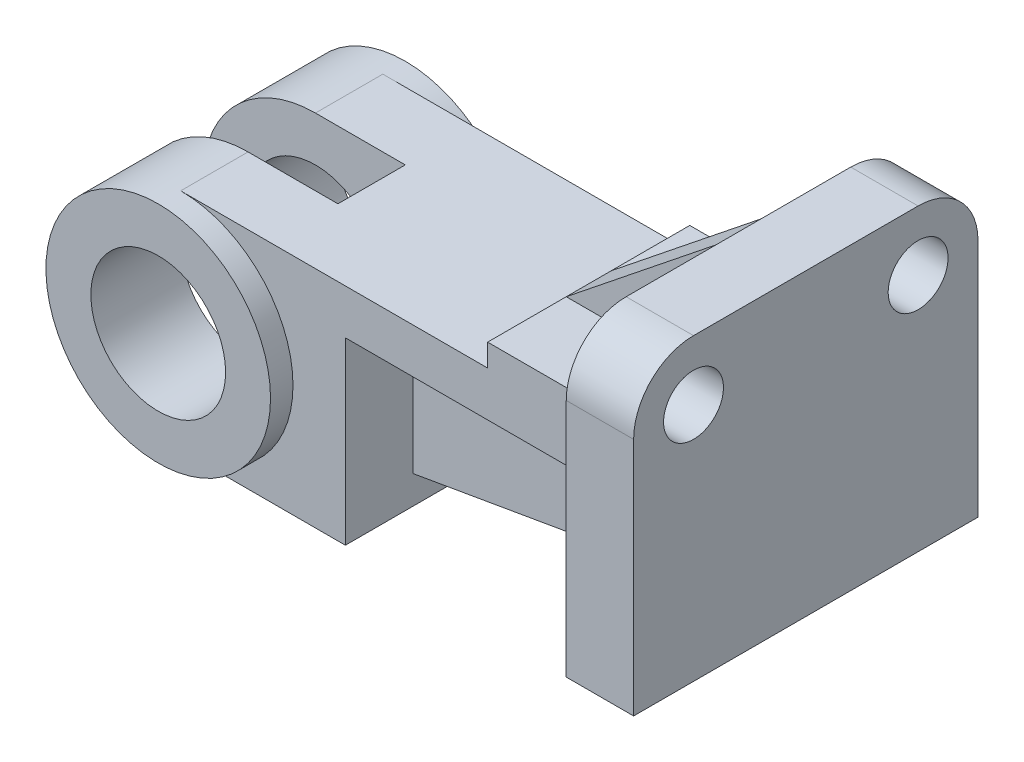
ISO-10303-21;
HEADER;
FILE_DESCRIPTION(('STEP AP214'),'2;1');
FILE_NAME('part.step','',(''),(''),'','','');
FILE_SCHEMA(('AUTOMOTIVE_DESIGN { 1 0 10303 214 1 1 1 1 }'));
ENDSEC;
DATA;
#1=APPLICATION_CONTEXT('core data for automotive mechanical design processes');
#2=APPLICATION_PROTOCOL_DEFINITION('international standard','automotive_design',2000,#1);
#3=PRODUCT_CONTEXT('',#1,'mechanical');
#4=PRODUCT('Part','Part','',(#3));
#5=PRODUCT_RELATED_PRODUCT_CATEGORY('part','',(#4));
#6=PRODUCT_DEFINITION_FORMATION('','',#4);
#7=PRODUCT_DEFINITION_CONTEXT('part definition',#1,'design');
#8=PRODUCT_DEFINITION('design','',#6,#7);
#9=PRODUCT_DEFINITION_SHAPE('','',#8);
#10=(LENGTH_UNIT() NAMED_UNIT(*) SI_UNIT(.MILLI.,.METRE.));
#11=(NAMED_UNIT(*) PLANE_ANGLE_UNIT() SI_UNIT($,.RADIAN.));
#12=(NAMED_UNIT(*) SI_UNIT($,.STERADIAN.) SOLID_ANGLE_UNIT());
#13=UNCERTAINTY_MEASURE_WITH_UNIT(LENGTH_MEASURE(1.E-05),#10,'distance_accuracy_value','');
#14=(GEOMETRIC_REPRESENTATION_CONTEXT(3) GLOBAL_UNCERTAINTY_ASSIGNED_CONTEXT((#13)) GLOBAL_UNIT_ASSIGNED_CONTEXT((#10,
#11,#12)) REPRESENTATION_CONTEXT('',''));
#15=CARTESIAN_POINT('',(0.,0.,0.));
#16=DIRECTION('',(0.,0.,1.));
#17=DIRECTION('',(1.,0.,0.));
#18=AXIS2_PLACEMENT_3D('',#15,#16,#17);
#19=CARTESIAN_POINT('',(104.,0.,-74.));
#20=DIRECTION('',(-1.,0.,0.));
#21=DIRECTION('',(0.,0.,1.));
#22=AXIS2_PLACEMENT_3D('',#19,#20,#21);
#23=PLANE('',#22);
#24=DIRECTION('',(0.,0.,1.));
#25=VECTOR('',#24,1.);
#26=CARTESIAN_POINT('',(104.,18.,-74.));
#27=LINE('',#26,#25);
#28=CARTESIAN_POINT('',(104.,18.,0.));
#29=VERTEX_POINT('',#28);
#30=CARTESIAN_POINT('',(104.,18.,18.));
#31=VERTEX_POINT('',#30);
#32=EDGE_CURVE('E277',#29,#31,#27,.T.);
#33=ORIENTED_EDGE('',*,*,#32,.F.);
#34=DIRECTION('',(0.,-1.,0.));
#35=VECTOR('',#34,1.);
#36=CARTESIAN_POINT('',(104.,0.,0.));
#37=LINE('',#36,#35);
#38=CARTESIAN_POINT('',(104.,-12.,0.));
#39=VERTEX_POINT('',#38);
#40=EDGE_CURVE('E57',#29,#39,#37,.T.);
#41=ORIENTED_EDGE('',*,*,#40,.T.);
#42=DIRECTION('',(0.,0.,1.));
#43=VECTOR('',#42,1.);
#44=CARTESIAN_POINT('',(104.,-12.,-74.));
#45=LINE('',#44,#43);
#46=CARTESIAN_POINT('',(104.,-12.,18.));
#47=VERTEX_POINT('',#46);
#48=EDGE_CURVE('E284',#39,#47,#45,.T.);
#49=ORIENTED_EDGE('',*,*,#48,.T.);
#50=DIRECTION('',(0.,-1.,0.));
#51=VECTOR('',#50,1.);
#52=CARTESIAN_POINT('',(104.,0.,18.));
#53=LINE('',#52,#51);
#54=EDGE_CURVE('E263',#31,#47,#53,.T.);
#55=ORIENTED_EDGE('',*,*,#54,.F.);
#56=EDGE_LOOP('',(#33,#41,#49,#55));
#57=FACE_BOUND('',#56,.T.);
#58=ADVANCED_FACE('F37',(#57),#23,.T.);
#59=CARTESIAN_POINT('',(0.,18.,-74.));
#60=DIRECTION('',(0.,-1.,0.));
#61=DIRECTION('',(0.,0.,-1.));
#62=AXIS2_PLACEMENT_3D('',#59,#60,#61);
#63=PLANE('',#62);
#64=DIRECTION('',(0.,0.,1.));
#65=VECTOR('',#64,1.);
#66=CARTESIAN_POINT('',(44.,18.,-74.));
#67=LINE('',#66,#65);
#68=CARTESIAN_POINT('',(44.,18.,0.));
#69=VERTEX_POINT('',#68);
#70=CARTESIAN_POINT('',(44.,18.,18.));
#71=VERTEX_POINT('',#70);
#72=EDGE_CURVE('E286',#69,#71,#67,.T.);
#73=ORIENTED_EDGE('',*,*,#72,.F.);
#74=DIRECTION('',(1.,0.,0.));
#75=VECTOR('',#74,1.);
#76=CARTESIAN_POINT('',(0.,18.,0.));
#77=LINE('',#76,#75);
#78=EDGE_CURVE('E232',#69,#29,#77,.T.);
#79=ORIENTED_EDGE('',*,*,#78,.T.);
#80=ORIENTED_EDGE('',*,*,#32,.T.);
#81=DIRECTION('',(1.,0.,0.));
#82=VECTOR('',#81,1.);
#83=CARTESIAN_POINT('',(0.,18.,18.));
#84=LINE('',#83,#82);
#85=EDGE_CURVE('E267',#71,#31,#84,.T.);
#86=ORIENTED_EDGE('',*,*,#85,.F.);
#87=EDGE_LOOP('',(#73,#79,#80,#86));
#88=FACE_BOUND('',#87,.T.);
#89=ADVANCED_FACE('F496',(#88),#63,.T.);
#90=CARTESIAN_POINT('',(122.,-30.,-36.));
#91=DIRECTION('',(0.,-1.,0.));
#92=DIRECTION('',(0.,0.,-1.));
#93=AXIS2_PLACEMENT_3D('',#90,#91,#92);
#94=PLANE('',#93);
#95=DIRECTION('',(1.,0.,0.));
#96=VECTOR('',#95,1.);
#97=CARTESIAN_POINT('',(122.,-30.,-36.));
#98=LINE('',#97,#96);
#99=CARTESIAN_POINT('',(0.,-30.,-36.));
#100=VERTEX_POINT('',#99);
#101=CARTESIAN_POINT('',(44.,-30.,-36.));
#102=VERTEX_POINT('',#101);
#103=EDGE_CURVE('E416',#100,#102,#98,.T.);
#104=ORIENTED_EDGE('',*,*,#103,.T.);
#105=DIRECTION('',(0.,0.,1.));
#106=VECTOR('',#105,1.);
#107=CARTESIAN_POINT('',(44.,-30.,-74.));
#108=LINE('',#107,#106);
#109=CARTESIAN_POINT('',(44.,-30.,18.));
#110=VERTEX_POINT('',#109);
#111=EDGE_CURVE('E281',#102,#110,#108,.T.);
#112=ORIENTED_EDGE('',*,*,#111,.T.);
#113=DIRECTION('',(1.,0.,0.));
#114=VECTOR('',#113,1.);
#115=CARTESIAN_POINT('',(122.,-30.,18.));
#116=LINE('',#115,#114);
#117=CARTESIAN_POINT('',(0.,-30.,18.));
#118=VERTEX_POINT('',#117);
#119=EDGE_CURVE('E426',#118,#110,#116,.T.);
#120=ORIENTED_EDGE('',*,*,#119,.F.);
#121=DIRECTION('',(0.,0.,1.));
#122=VECTOR('',#121,1.);
#123=CARTESIAN_POINT('',(0.,-30.,-36.));
#124=LINE('',#123,#122);
#125=CARTESIAN_POINT('',(0.,-30.,0.));
#126=VERTEX_POINT('',#125);
#127=EDGE_CURVE('E424',#126,#118,#124,.T.);
#128=ORIENTED_EDGE('',*,*,#127,.F.);
#129=DIRECTION('',(-1.,0.,0.));
#130=VECTOR('',#129,1.);
#131=CARTESIAN_POINT('',(122.,-30.,0.));
#132=LINE('',#131,#130);
#133=CARTESIAN_POINT('',(24.,-30.,0.));
#134=VERTEX_POINT('',#133);
#135=EDGE_CURVE('E446',#134,#126,#132,.T.);
#136=ORIENTED_EDGE('',*,*,#135,.F.);
#137=DIRECTION('',(0.,0.,1.));
#138=VECTOR('',#137,1.);
#139=CARTESIAN_POINT('',(24.,-30.,-36.));
#140=LINE('',#139,#138);
#141=CARTESIAN_POINT('',(24.,-30.,-18.));
#142=VERTEX_POINT('',#141);
#143=EDGE_CURVE('E397',#142,#134,#140,.T.);
#144=ORIENTED_EDGE('',*,*,#143,.F.);
#145=DIRECTION('',(1.,0.,0.));
#146=VECTOR('',#145,1.);
#147=CARTESIAN_POINT('',(122.,-30.,-18.));
#148=LINE('',#147,#146);
#149=CARTESIAN_POINT('',(0.,-30.,-18.));
#150=VERTEX_POINT('',#149);
#151=EDGE_CURVE('E395',#150,#142,#148,.T.);
#152=ORIENTED_EDGE('',*,*,#151,.F.);
#153=EDGE_CURVE('E439',#100,#150,#124,.T.);
#154=ORIENTED_EDGE('',*,*,#153,.F.);
#155=EDGE_LOOP('',(#104,#112,#120,#128,#136,#144,#152,#154));
#156=FACE_BOUND('',#155,.T.);
#157=ADVANCED_FACE('F502',(#156),#94,.T.);
#158=CARTESIAN_POINT('',(0.,36.,0.));
#159=DIRECTION('',(0.,-1.,0.));
#160=DIRECTION('',(0.,0.,-1.));
#161=AXIS2_PLACEMENT_3D('',#158,#159,#160);
#162=PLANE('',#161);
#163=DIRECTION('',(0.,0.,1.));
#164=VECTOR('',#163,1.);
#165=CARTESIAN_POINT('',(82.,36.,18.));
#166=LINE('',#165,#164);
#167=CARTESIAN_POINT('',(82.,36.,-3.));
#168=VERTEX_POINT('',#167);
#169=CARTESIAN_POINT('',(82.,36.,18.));
#170=VERTEX_POINT('',#169);
#171=EDGE_CURVE('E359',#168,#170,#166,.T.);
#172=ORIENTED_EDGE('',*,*,#171,.T.);
#173=DIRECTION('',(1.,0.,0.));
#174=VECTOR('',#173,1.);
#175=CARTESIAN_POINT('',(122.,36.,18.));
#176=LINE('',#175,#174);
#177=CARTESIAN_POINT('',(122.,36.,18.));
#178=VERTEX_POINT('',#177);
#179=EDGE_CURVE('E361',#170,#178,#176,.T.);
#180=ORIENTED_EDGE('',*,*,#179,.T.);
#181=DIRECTION('',(0.,0.,-1.));
#182=VECTOR('',#181,1.);
#183=CARTESIAN_POINT('',(122.,36.,-36.));
#184=LINE('',#183,#182);
#185=CARTESIAN_POINT('',(122.,36.,-3.));
#186=VERTEX_POINT('',#185);
#187=EDGE_CURVE('E355',#178,#186,#184,.T.);
#188=ORIENTED_EDGE('',*,*,#187,.T.);
#189=DIRECTION('',(1.,0.,0.));
#190=VECTOR('',#189,1.);
#191=CARTESIAN_POINT('',(0.,36.,-3.));
#192=LINE('',#191,#190);
#193=EDGE_CURVE('E302',#168,#186,#192,.T.);
#194=ORIENTED_EDGE('',*,*,#193,.F.);
#195=EDGE_LOOP('',(#172,#180,#188,#194));
#196=FACE_BOUND('',#195,.T.);
#197=ADVANCED_FACE('F611',(#196),#162,.F.);
#198=CARTESIAN_POINT('',(122.,-12.,-55.));
#199=DIRECTION('',(1.,0.,0.));
#200=DIRECTION('',(0.,0.,-1.));
#201=AXIS2_PLACEMENT_3D('',#198,#199,#200);
#202=PLANE('',#201);
#203=DIRECTION('',(0.,1.,0.));
#204=VECTOR('',#203,1.);
#205=CARTESIAN_POINT('',(122.,-12.,-3.));
#206=LINE('',#205,#204);
#207=CARTESIAN_POINT('',(122.,68.,-3.));
#208=VERTEX_POINT('',#207);
#209=EDGE_CURVE('E301',#186,#208,#206,.T.);
#210=ORIENTED_EDGE('',*,*,#209,.F.);
#211=ORIENTED_EDGE('',*,*,#187,.F.);
#212=DIRECTION('',(0.,1.,0.));
#213=VECTOR('',#212,1.);
#214=CARTESIAN_POINT('',(122.,30.,18.));
#215=LINE('',#214,#213);
#216=CARTESIAN_POINT('',(122.,-12.,18.));
#217=VERTEX_POINT('',#216);
#218=EDGE_CURVE('E431',#217,#178,#215,.T.);
#219=ORIENTED_EDGE('',*,*,#218,.F.);
#220=DIRECTION('',(0.,0.,1.));
#221=VECTOR('',#220,1.);
#222=CARTESIAN_POINT('',(122.,-12.,-55.));
#223=LINE('',#222,#221);
#224=CARTESIAN_POINT('',(122.,-12.,37.));
#225=VERTEX_POINT('',#224);
#226=EDGE_CURVE('E347',#217,#225,#223,.T.);
#227=ORIENTED_EDGE('',*,*,#226,.T.);
#228=DIRECTION('',(0.,1.,0.));
#229=VECTOR('',#228,1.);
#230=CARTESIAN_POINT('',(122.,-12.,37.));
#231=LINE('',#230,#229);
#232=CARTESIAN_POINT('',(122.,52.,37.));
#233=VERTEX_POINT('',#232);
#234=EDGE_CURVE('E336',#225,#233,#231,.T.);
#235=ORIENTED_EDGE('',*,*,#234,.T.);
#236=CARTESIAN_POINT('',(122.,52.,21.));
#237=DIRECTION('',(1.,0.,0.));
#238=DIRECTION('',(0.,0.,-1.));
#239=AXIS2_PLACEMENT_3D('',#236,#237,#238);
#240=CIRCLE('',#239,16.);
#241=CARTESIAN_POINT('',(122.,68.,21.));
#242=VERTEX_POINT('',#241);
#243=EDGE_CURVE('E463',#233,#242,#240,.F.);
#244=ORIENTED_EDGE('',*,*,#243,.T.);
#245=DIRECTION('',(0.,0.,1.));
#246=VECTOR('',#245,1.);
#247=CARTESIAN_POINT('',(122.,68.,-55.));
#248=LINE('',#247,#246);
#249=EDGE_CURVE('E346',#208,#242,#248,.T.);
#250=ORIENTED_EDGE('',*,*,#249,.F.);
#251=EDGE_LOOP('',(#210,#211,#219,#227,#235,#244,#250));
#252=FACE_BOUND('',#251,.T.);
#253=CARTESIAN_POINT('',(122.,52.,21.));
#254=DIRECTION('',(-1.,0.,0.));
#255=DIRECTION('',(0.,0.,1.));
#256=AXIS2_PLACEMENT_3D('',#253,#254,#255);
#257=CIRCLE('',#256,8.);
#258=CARTESIAN_POINT('',(122.,52.,29.));
#259=VERTEX_POINT('',#258);
#260=EDGE_CURVE('E316',#259,#259,#257,.T.);
#261=ORIENTED_EDGE('',*,*,#260,.F.);
#262=EDGE_LOOP('',(#261));
#263=FACE_BOUND('',#262,.T.);
#264=ADVANCED_FACE('F642',(#252,#263),#202,.F.);
#265=CARTESIAN_POINT('',(0.,30.,-36.));
#266=DIRECTION('',(0.,1.,0.));
#267=DIRECTION('',(0.,0.,1.));
#268=AXIS2_PLACEMENT_3D('',#265,#266,#267);
#269=PLANE('',#268);
#270=DIRECTION('',(-1.,0.,0.));
#271=VECTOR('',#270,1.);
#272=CARTESIAN_POINT('',(24.,30.,-18.));
#273=LINE('',#272,#271);
#274=CARTESIAN_POINT('',(24.,30.,-18.));
#275=VERTEX_POINT('',#274);
#276=CARTESIAN_POINT('',(0.,30.,-18.));
#277=VERTEX_POINT('',#276);
#278=EDGE_CURVE('E389',#275,#277,#273,.T.);
#279=ORIENTED_EDGE('',*,*,#278,.F.);
#280=DIRECTION('',(0.,0.,-1.));
#281=VECTOR('',#280,1.);
#282=CARTESIAN_POINT('',(24.,30.,0.));
#283=LINE('',#282,#281);
#284=CARTESIAN_POINT('',(24.,30.,0.));
#285=VERTEX_POINT('',#284);
#286=EDGE_CURVE('E383',#285,#275,#283,.T.);
#287=ORIENTED_EDGE('',*,*,#286,.F.);
#288=DIRECTION('',(1.,0.,0.));
#289=VECTOR('',#288,1.);
#290=CARTESIAN_POINT('',(0.,30.,0.));
#291=LINE('',#290,#289);
#292=CARTESIAN_POINT('',(0.,30.,0.));
#293=VERTEX_POINT('',#292);
#294=EDGE_CURVE('E385',#293,#285,#291,.T.);
#295=ORIENTED_EDGE('',*,*,#294,.F.);
#296=DIRECTION('',(0.,0.,1.));
#297=VECTOR('',#296,1.);
#298=CARTESIAN_POINT('',(0.,30.,-36.));
#299=LINE('',#298,#297);
#300=CARTESIAN_POINT('',(0.,30.,18.));
#301=VERTEX_POINT('',#300);
#302=EDGE_CURVE('E437',#293,#301,#299,.T.);
#303=ORIENTED_EDGE('',*,*,#302,.T.);
#304=DIRECTION('',(-1.,0.,0.));
#305=VECTOR('',#304,1.);
#306=CARTESIAN_POINT('',(0.,30.,18.));
#307=LINE('',#306,#305);
#308=CARTESIAN_POINT('',(82.,30.,18.));
#309=VERTEX_POINT('',#308);
#310=EDGE_CURVE('E417',#309,#301,#307,.T.);
#311=ORIENTED_EDGE('',*,*,#310,.F.);
#312=DIRECTION('',(0.,0.,1.));
#313=VECTOR('',#312,1.);
#314=CARTESIAN_POINT('',(82.,30.,18.));
#315=LINE('',#314,#313);
#316=CARTESIAN_POINT('',(82.,30.,-36.));
#317=VERTEX_POINT('',#316);
#318=EDGE_CURVE('E353',#317,#309,#315,.T.);
#319=ORIENTED_EDGE('',*,*,#318,.F.);
#320=DIRECTION('',(-1.,0.,0.));
#321=VECTOR('',#320,1.);
#322=CARTESIAN_POINT('',(0.,30.,-36.));
#323=LINE('',#322,#321);
#324=CARTESIAN_POINT('',(0.,30.,-36.));
#325=VERTEX_POINT('',#324);
#326=EDGE_CURVE('E421',#317,#325,#323,.T.);
#327=ORIENTED_EDGE('',*,*,#326,.T.);
#328=EDGE_CURVE('E434',#325,#277,#299,.T.);
#329=ORIENTED_EDGE('',*,*,#328,.T.);
#330=EDGE_LOOP('',(#279,#287,#295,#303,#311,#319,#327,#329));
#331=FACE_BOUND('',#330,.T.);
#332=ADVANCED_FACE('F646',(#331),#269,.T.);
#333=CARTESIAN_POINT('',(0.,0.,0.));
#334=DIRECTION('',(0.,0.,1.));
#335=DIRECTION('',(1.,0.,0.));
#336=AXIS2_PLACEMENT_3D('',#333,#334,#335);
#337=PLANE('',#336);
#338=ORIENTED_EDGE('',*,*,#135,.T.);
#339=CARTESIAN_POINT('',(0.,0.,0.));
#340=DIRECTION('',(0.,0.,1.));
#341=DIRECTION('',(1.,0.,0.));
#342=AXIS2_PLACEMENT_3D('',#339,#340,#341);
#343=CIRCLE('',#342,30.);
#344=EDGE_CURVE('E448',#293,#126,#343,.T.);
#345=ORIENTED_EDGE('',*,*,#344,.F.);
#346=ORIENTED_EDGE('',*,*,#294,.T.);
#347=DIRECTION('',(0.,1.,0.));
#348=VECTOR('',#347,1.);
#349=CARTESIAN_POINT('',(24.,-66.,0.));
#350=LINE('',#349,#348);
#351=EDGE_CURVE('E388',#134,#285,#350,.T.);
#352=ORIENTED_EDGE('',*,*,#351,.F.);
#353=EDGE_LOOP('',(#338,#345,#346,#352));
#354=FACE_BOUND('',#353,.T.);
#355=CARTESIAN_POINT('',(0.,0.,0.));
#356=DIRECTION('',(0.,0.,1.));
#357=DIRECTION('',(1.,0.,0.));
#358=AXIS2_PLACEMENT_3D('',#355,#356,#357);
#359=CIRCLE('',#358,18.);
#360=CARTESIAN_POINT('',(18.,0.,0.));
#361=VERTEX_POINT('',#360);
#362=EDGE_CURVE('E444',#361,#361,#359,.T.);
#363=ORIENTED_EDGE('',*,*,#362,.T.);
#364=EDGE_LOOP('',(#363));
#365=FACE_BOUND('',#364,.T.);
#366=ADVANCED_FACE('F747',(#354,#365),#337,.F.);
#367=CARTESIAN_POINT('',(0.,0.,-18.));
#368=DIRECTION('',(0.,0.,-1.));
#369=DIRECTION('',(-1.,0.,0.));
#370=AXIS2_PLACEMENT_3D('',#367,#368,#369);
#371=PLANE('',#370);
#372=CARTESIAN_POINT('',(0.,0.,-18.));
#373=DIRECTION('',(0.,0.,-1.));
#374=DIRECTION('',(-1.,0.,0.));
#375=AXIS2_PLACEMENT_3D('',#372,#373,#374);
#376=CIRCLE('',#375,18.);
#377=CARTESIAN_POINT('',(-18.,0.,-18.));
#378=VERTEX_POINT('',#377);
#379=EDGE_CURVE('E398',#378,#378,#376,.T.);
#380=ORIENTED_EDGE('',*,*,#379,.T.);
#381=EDGE_LOOP('',(#380));
#382=FACE_BOUND('',#381,.T.);
#383=CARTESIAN_POINT('',(0.,0.,-18.));
#384=DIRECTION('',(0.,0.,-1.));
#385=DIRECTION('',(-1.,0.,0.));
#386=AXIS2_PLACEMENT_3D('',#383,#384,#385);
#387=CIRCLE('',#386,30.);
#388=EDGE_CURVE('E401',#150,#277,#387,.T.);
#389=ORIENTED_EDGE('',*,*,#388,.F.);
#390=ORIENTED_EDGE('',*,*,#151,.T.);
#391=DIRECTION('',(0.,1.,0.));
#392=VECTOR('',#391,1.);
#393=CARTESIAN_POINT('',(24.,-66.,-18.));
#394=LINE('',#393,#392);
#395=EDGE_CURVE('E394',#142,#275,#394,.T.);
#396=ORIENTED_EDGE('',*,*,#395,.T.);
#397=ORIENTED_EDGE('',*,*,#278,.T.);
#398=EDGE_LOOP('',(#389,#390,#396,#397));
#399=FACE_BOUND('',#398,.T.);
#400=ADVANCED_FACE('F769',(#382,#399),#371,.F.);
#401=CARTESIAN_POINT('',(0.,0.,24.));
#402=DIRECTION('',(0.,0.,-1.));
#403=DIRECTION('',(-1.,0.,0.));
#404=AXIS2_PLACEMENT_3D('',#401,#402,#403);
#405=CYLINDRICAL_SURFACE('',#404,30.);
#406=CARTESIAN_POINT('',(0.,0.,18.));
#407=DIRECTION('',(0.,0.,-1.));
#408=DIRECTION('',(1.,0.,0.));
#409=AXIS2_PLACEMENT_3D('',#406,#407,#408);
#410=CIRCLE('',#409,30.);
#411=EDGE_CURVE('E410',#301,#118,#410,.T.);
#412=ORIENTED_EDGE('',*,*,#411,.F.);
#413=ORIENTED_EDGE('',*,*,#302,.F.);
#414=ORIENTED_EDGE('',*,*,#344,.T.);
#415=ORIENTED_EDGE('',*,*,#127,.T.);
#416=EDGE_LOOP('',(#412,#413,#414,#415));
#417=FACE_BOUND('',#416,.T.);
#418=CARTESIAN_POINT('',(0.,0.,24.));
#419=DIRECTION('',(0.,0.,1.));
#420=DIRECTION('',(1.,0.,0.));
#421=AXIS2_PLACEMENT_3D('',#418,#419,#420);
#422=CIRCLE('',#421,30.);
#423=CARTESIAN_POINT('',(30.,0.,24.));
#424=VERTEX_POINT('',#423);
#425=EDGE_CURVE('E447',#424,#424,#422,.T.);
#426=ORIENTED_EDGE('',*,*,#425,.F.);
#427=EDGE_LOOP('',(#426));
#428=FACE_BOUND('',#427,.T.);
#429=ADVANCED_FACE('F785',(#417,#428),#405,.T.);
#430=CARTESIAN_POINT('',(0.,0.,24.));
#431=DIRECTION('',(0.,0.,1.));
#432=DIRECTION('',(1.,0.,0.));
#433=AXIS2_PLACEMENT_3D('',#430,#431,#432);
#434=PLANE('',#433);
#435=CARTESIAN_POINT('',(0.,0.,24.));
#436=DIRECTION('',(0.,0.,1.));
#437=DIRECTION('',(1.,0.,0.));
#438=AXIS2_PLACEMENT_3D('',#435,#436,#437);
#439=CIRCLE('',#438,18.);
#440=CARTESIAN_POINT('',(18.,0.,24.));
#441=VERTEX_POINT('',#440);
#442=EDGE_CURVE('E438',#441,#441,#439,.T.);
#443=ORIENTED_EDGE('',*,*,#442,.F.);
#444=EDGE_LOOP('',(#443));
#445=FACE_BOUND('',#444,.T.);
#446=ORIENTED_EDGE('',*,*,#425,.T.);
#447=EDGE_LOOP('',(#446));
#448=FACE_BOUND('',#447,.T.);
#449=ADVANCED_FACE('F870',(#445,#448),#434,.T.);
#450=CARTESIAN_POINT('',(0.,0.,-74.));
#451=DIRECTION('',(0.,0.,1.));
#452=DIRECTION('',(1.,0.,0.));
#453=AXIS2_PLACEMENT_3D('',#450,#451,#452);
#454=CYLINDRICAL_SURFACE('',#453,18.);
#455=ORIENTED_EDGE('',*,*,#442,.T.);
#456=EDGE_LOOP('',(#455));
#457=FACE_BOUND('',#456,.T.);
#458=ORIENTED_EDGE('',*,*,#362,.F.);
#459=EDGE_LOOP('',(#458));
#460=FACE_BOUND('',#459,.T.);
#461=ADVANCED_FACE('F814',(#457,#460),#454,.F.);
#462=CARTESIAN_POINT('',(0.,0.,-36.));
#463=DIRECTION('',(0.,0.,1.));
#464=DIRECTION('',(1.,0.,0.));
#465=AXIS2_PLACEMENT_3D('',#462,#463,#464);
#466=PLANE('',#465);
#467=DIRECTION('',(0.,1.,0.));
#468=VECTOR('',#467,1.);
#469=CARTESIAN_POINT('',(122.,30.,-36.));
#470=LINE('',#469,#468);
#471=CARTESIAN_POINT('',(122.,-12.,-36.));
#472=VERTEX_POINT('',#471);
#473=CARTESIAN_POINT('',(122.,36.,-36.));
#474=VERTEX_POINT('',#473);
#475=EDGE_CURVE('E420',#472,#474,#470,.T.);
#476=ORIENTED_EDGE('',*,*,#475,.F.);
#477=DIRECTION('',(-1.,0.,0.));
#478=VECTOR('',#477,1.);
#479=CARTESIAN_POINT('',(0.,-12.,-36.));
#480=LINE('',#479,#478);
#481=CARTESIAN_POINT('',(104.,-12.,-36.));
#482=VERTEX_POINT('',#481);
#483=EDGE_CURVE('E278',#472,#482,#480,.T.);
#484=ORIENTED_EDGE('',*,*,#483,.T.);
#485=DIRECTION('',(0.,-1.,0.));
#486=VECTOR('',#485,1.);
#487=CARTESIAN_POINT('',(104.,0.,-36.));
#488=LINE('',#487,#486);
#489=CARTESIAN_POINT('',(104.,18.,-36.));
#490=VERTEX_POINT('',#489);
#491=EDGE_CURVE('E298',#490,#482,#488,.T.);
#492=ORIENTED_EDGE('',*,*,#491,.F.);
#493=DIRECTION('',(1.,0.,0.));
#494=VECTOR('',#493,1.);
#495=CARTESIAN_POINT('',(0.,18.,-36.));
#496=LINE('',#495,#494);
#497=CARTESIAN_POINT('',(44.,18.,-36.));
#498=VERTEX_POINT('',#497);
#499=EDGE_CURVE('E292',#498,#490,#496,.T.);
#500=ORIENTED_EDGE('',*,*,#499,.F.);
#501=DIRECTION('',(0.,1.,0.));
#502=VECTOR('',#501,1.);
#503=CARTESIAN_POINT('',(44.,0.,-36.));
#504=LINE('',#503,#502);
#505=EDGE_CURVE('E295',#102,#498,#504,.T.);
#506=ORIENTED_EDGE('',*,*,#505,.F.);
#507=ORIENTED_EDGE('',*,*,#103,.F.);
#508=CARTESIAN_POINT('',(0.,0.,-36.));
#509=DIRECTION('',(0.,0.,-1.));
#510=DIRECTION('',(1.,0.,0.));
#511=AXIS2_PLACEMENT_3D('',#508,#509,#510);
#512=CIRCLE('',#511,30.);
#513=EDGE_CURVE('E415',#325,#100,#512,.T.);
#514=ORIENTED_EDGE('',*,*,#513,.F.);
#515=ORIENTED_EDGE('',*,*,#326,.F.);
#516=DIRECTION('',(0.,-1.,0.));
#517=VECTOR('',#516,1.);
#518=CARTESIAN_POINT('',(82.,36.,-36.));
#519=LINE('',#518,#517);
#520=CARTESIAN_POINT('',(82.,36.,-36.));
#521=VERTEX_POINT('',#520);
#522=EDGE_CURVE('E369',#521,#317,#519,.T.);
#523=ORIENTED_EDGE('',*,*,#522,.F.);
#524=DIRECTION('',(-1.,0.,0.));
#525=VECTOR('',#524,1.);
#526=CARTESIAN_POINT('',(82.,36.,-36.));
#527=LINE('',#526,#525);
#528=EDGE_CURVE('E357',#474,#521,#527,.T.);
#529=ORIENTED_EDGE('',*,*,#528,.F.);
#530=EDGE_LOOP('',(#476,#484,#492,#500,#506,#507,#514,#515,#523,#529));
#531=FACE_BOUND('',#530,.T.);
#532=ADVANCED_FACE('F530',(#531),#466,.F.);
#533=CARTESIAN_POINT('',(0.,0.,18.));
#534=DIRECTION('',(0.,0.,1.));
#535=DIRECTION('',(1.,0.,0.));
#536=AXIS2_PLACEMENT_3D('',#533,#534,#535);
#537=PLANE('',#536);
#538=DIRECTION('',(-1.,0.,0.));
#539=VECTOR('',#538,1.);
#540=CARTESIAN_POINT('',(0.,-12.,18.));
#541=LINE('',#540,#539);
#542=EDGE_CURVE('E271',#217,#47,#541,.T.);
#543=ORIENTED_EDGE('',*,*,#542,.F.);
#544=ORIENTED_EDGE('',*,*,#218,.T.);
#545=ORIENTED_EDGE('',*,*,#179,.F.);
#546=DIRECTION('',(0.,-1.,0.));
#547=VECTOR('',#546,1.);
#548=CARTESIAN_POINT('',(82.,36.,18.));
#549=LINE('',#548,#547);
#550=EDGE_CURVE('E366',#170,#309,#549,.T.);
#551=ORIENTED_EDGE('',*,*,#550,.T.);
#552=ORIENTED_EDGE('',*,*,#310,.T.);
#553=ORIENTED_EDGE('',*,*,#411,.T.);
#554=ORIENTED_EDGE('',*,*,#119,.T.);
#555=DIRECTION('',(0.,1.,0.));
#556=VECTOR('',#555,1.);
#557=CARTESIAN_POINT('',(44.,0.,18.));
#558=LINE('',#557,#556);
#559=EDGE_CURVE('E270',#110,#71,#558,.T.);
#560=ORIENTED_EDGE('',*,*,#559,.T.);
#561=ORIENTED_EDGE('',*,*,#85,.T.);
#562=ORIENTED_EDGE('',*,*,#54,.T.);
#563=EDGE_LOOP('',(#543,#544,#545,#551,#552,#553,#554,#560,#561,#562));
#564=FACE_BOUND('',#563,.T.);
#565=ADVANCED_FACE('F804',(#564),#537,.T.);
#566=CARTESIAN_POINT('',(0.,0.,-42.));
#567=DIRECTION('',(0.,0.,1.));
#568=DIRECTION('',(1.,0.,0.));
#569=AXIS2_PLACEMENT_3D('',#566,#567,#568);
#570=CYLINDRICAL_SURFACE('',#569,30.);
#571=CARTESIAN_POINT('',(0.,0.,-42.));
#572=DIRECTION('',(0.,0.,-1.));
#573=DIRECTION('',(-1.,0.,0.));
#574=AXIS2_PLACEMENT_3D('',#571,#572,#573);
#575=CIRCLE('',#574,30.);
#576=CARTESIAN_POINT('',(-30.,0.,-42.));
#577=VERTEX_POINT('',#576);
#578=EDGE_CURVE('E404',#577,#577,#575,.T.);
#579=ORIENTED_EDGE('',*,*,#578,.F.);
#580=EDGE_LOOP('',(#579));
#581=FACE_BOUND('',#580,.T.);
#582=ORIENTED_EDGE('',*,*,#388,.T.);
#583=ORIENTED_EDGE('',*,*,#328,.F.);
#584=ORIENTED_EDGE('',*,*,#513,.T.);
#585=ORIENTED_EDGE('',*,*,#153,.T.);
#586=EDGE_LOOP('',(#582,#583,#584,#585));
#587=FACE_BOUND('',#586,.T.);
#588=ADVANCED_FACE('F802',(#581,#587),#570,.T.);
#589=CARTESIAN_POINT('',(0.,0.,-42.));
#590=DIRECTION('',(0.,0.,-1.));
#591=DIRECTION('',(-1.,0.,0.));
#592=AXIS2_PLACEMENT_3D('',#589,#590,#591);
#593=PLANE('',#592);
#594=CARTESIAN_POINT('',(0.,0.,-42.));
#595=DIRECTION('',(0.,0.,-1.));
#596=DIRECTION('',(-1.,0.,0.));
#597=AXIS2_PLACEMENT_3D('',#594,#595,#596);
#598=CIRCLE('',#597,18.);
#599=CARTESIAN_POINT('',(-18.,0.,-42.));
#600=VERTEX_POINT('',#599);
#601=EDGE_CURVE('E400',#600,#600,#598,.T.);
#602=ORIENTED_EDGE('',*,*,#601,.F.);
#603=EDGE_LOOP('',(#602));
#604=FACE_BOUND('',#603,.T.);
#605=ORIENTED_EDGE('',*,*,#578,.T.);
#606=EDGE_LOOP('',(#605));
#607=FACE_BOUND('',#606,.T.);
#608=ADVANCED_FACE('F829',(#604,#607),#593,.T.);
#609=CARTESIAN_POINT('',(0.,0.,-74.));
#610=DIRECTION('',(0.,0.,1.));
#611=DIRECTION('',(1.,0.,0.));
#612=AXIS2_PLACEMENT_3D('',#609,#610,#611);
#613=CYLINDRICAL_SURFACE('',#612,18.);
#614=ORIENTED_EDGE('',*,*,#601,.T.);
#615=EDGE_LOOP('',(#614));
#616=FACE_BOUND('',#615,.T.);
#617=ORIENTED_EDGE('',*,*,#379,.F.);
#618=EDGE_LOOP('',(#617));
#619=FACE_BOUND('',#618,.T.);
#620=ADVANCED_FACE('F793',(#616,#619),#613,.F.);
#621=CARTESIAN_POINT('',(24.,-66.,0.));
#622=DIRECTION('',(1.,0.,0.));
#623=DIRECTION('',(0.,0.,-1.));
#624=AXIS2_PLACEMENT_3D('',#621,#622,#623);
#625=PLANE('',#624);
#626=ORIENTED_EDGE('',*,*,#351,.T.);
#627=ORIENTED_EDGE('',*,*,#286,.T.);
#628=ORIENTED_EDGE('',*,*,#395,.F.);
#629=ORIENTED_EDGE('',*,*,#143,.T.);
#630=EDGE_LOOP('',(#626,#627,#628,#629));
#631=FACE_BOUND('',#630,.T.);
#632=ADVANCED_FACE('F736',(#631),#625,.F.);
#633=CARTESIAN_POINT('',(82.,36.,18.));
#634=DIRECTION('',(1.,0.,0.));
#635=DIRECTION('',(0.,0.,-1.));
#636=AXIS2_PLACEMENT_3D('',#633,#634,#635);
#637=PLANE('',#636);
#638=ORIENTED_EDGE('',*,*,#318,.T.);
#639=ORIENTED_EDGE('',*,*,#550,.F.);
#640=ORIENTED_EDGE('',*,*,#171,.F.);
#641=DIRECTION('',(0.,0.,-1.));
#642=VECTOR('',#641,1.);
#643=CARTESIAN_POINT('',(82.,36.,0.));
#644=LINE('',#643,#642);
#645=CARTESIAN_POINT('',(82.,36.,-15.));
#646=VERTEX_POINT('',#645);
#647=EDGE_CURVE('E314',#168,#646,#644,.T.);
#648=ORIENTED_EDGE('',*,*,#647,.T.);
#649=EDGE_CURVE('E363',#521,#646,#166,.T.);
#650=ORIENTED_EDGE('',*,*,#649,.F.);
#651=ORIENTED_EDGE('',*,*,#522,.T.);
#652=EDGE_LOOP('',(#638,#639,#640,#648,#650,#651));
#653=FACE_BOUND('',#652,.T.);
#654=ADVANCED_FACE('F729',(#653),#637,.F.);
#655=ORIENTED_EDGE('',*,*,#649,.T.);
#656=DIRECTION('',(1.,0.,0.));
#657=VECTOR('',#656,1.);
#658=CARTESIAN_POINT('',(0.,36.,-15.));
#659=LINE('',#658,#657);
#660=CARTESIAN_POINT('',(122.,36.,-15.));
#661=VERTEX_POINT('',#660);
#662=EDGE_CURVE('E309',#646,#661,#659,.T.);
#663=ORIENTED_EDGE('',*,*,#662,.T.);
#664=EDGE_CURVE('E356',#661,#474,#184,.T.);
#665=ORIENTED_EDGE('',*,*,#664,.T.);
#666=ORIENTED_EDGE('',*,*,#528,.T.);
#667=EDGE_LOOP('',(#655,#663,#665,#666));
#668=FACE_BOUND('',#667,.T.);
#669=ADVANCED_FACE('F600',(#668),#162,.F.);
#670=CARTESIAN_POINT('',(140.,-12.,-55.));
#671=DIRECTION('',(0.,1.,0.));
#672=DIRECTION('',(0.,0.,1.));
#673=AXIS2_PLACEMENT_3D('',#670,#671,#672);
#674=PLANE('',#673);
#675=DIRECTION('',(0.,0.,1.));
#676=VECTOR('',#675,1.);
#677=CARTESIAN_POINT('',(140.,-12.,-55.));
#678=LINE('',#677,#676);
#679=CARTESIAN_POINT('',(140.,-12.,-55.));
#680=VERTEX_POINT('',#679);
#681=CARTESIAN_POINT('',(140.,-12.,37.));
#682=VERTEX_POINT('',#681);
#683=EDGE_CURVE('E333',#680,#682,#678,.T.);
#684=ORIENTED_EDGE('',*,*,#683,.T.);
#685=DIRECTION('',(-1.,0.,0.));
#686=VECTOR('',#685,1.);
#687=CARTESIAN_POINT('',(140.,-12.,37.));
#688=LINE('',#687,#686);
#689=EDGE_CURVE('E335',#682,#225,#688,.T.);
#690=ORIENTED_EDGE('',*,*,#689,.T.);
#691=ORIENTED_EDGE('',*,*,#226,.F.);
#692=ORIENTED_EDGE('',*,*,#542,.T.);
#693=ORIENTED_EDGE('',*,*,#48,.F.);
#694=DIRECTION('',(0.,0.,-1.));
#695=VECTOR('',#694,1.);
#696=CARTESIAN_POINT('',(104.,-12.,-74.));
#697=LINE('',#696,#695);
#698=CARTESIAN_POINT('',(104.,-12.,-18.));
#699=VERTEX_POINT('',#698);
#700=EDGE_CURVE('E244',#699,#39,#697,.F.);
#701=ORIENTED_EDGE('',*,*,#700,.F.);
#702=EDGE_CURVE('E280',#482,#699,#45,.T.);
#703=ORIENTED_EDGE('',*,*,#702,.F.);
#704=ORIENTED_EDGE('',*,*,#483,.F.);
#705=CARTESIAN_POINT('',(122.,-12.,-55.));
#706=VERTEX_POINT('',#705);
#707=EDGE_CURVE('E351',#706,#472,#223,.T.);
#708=ORIENTED_EDGE('',*,*,#707,.F.);
#709=DIRECTION('',(-1.,0.,0.));
#710=VECTOR('',#709,1.);
#711=CARTESIAN_POINT('',(140.,-12.,-55.));
#712=LINE('',#711,#710);
#713=EDGE_CURVE('E323',#680,#706,#712,.T.);
#714=ORIENTED_EDGE('',*,*,#713,.F.);
#715=EDGE_LOOP('',(#684,#690,#691,#692,#693,#701,#703,#704,#708,#714));
#716=FACE_BOUND('',#715,.T.);
#717=ADVANCED_FACE('F535',(#716),#674,.F.);
#718=CARTESIAN_POINT('',(122.,52.,-39.));
#719=DIRECTION('',(-1.,0.,0.));
#720=DIRECTION('',(0.,0.,1.));
#721=AXIS2_PLACEMENT_3D('',#718,#719,#720);
#722=CIRCLE('',#721,8.);
#723=CARTESIAN_POINT('',(122.,52.,-31.));
#724=VERTEX_POINT('',#723);
#725=EDGE_CURVE('E319',#724,#724,#722,.T.);
#726=ORIENTED_EDGE('',*,*,#725,.F.);
#727=EDGE_LOOP('',(#726));
#728=FACE_BOUND('',#727,.T.);
#729=ORIENTED_EDGE('',*,*,#475,.T.);
#730=ORIENTED_EDGE('',*,*,#664,.F.);
#731=DIRECTION('',(0.,1.,0.));
#732=VECTOR('',#731,1.);
#733=CARTESIAN_POINT('',(122.,-12.,-15.));
#734=LINE('',#733,#732);
#735=CARTESIAN_POINT('',(122.,68.,-15.));
#736=VERTEX_POINT('',#735);
#737=EDGE_CURVE('E310',#661,#736,#734,.T.);
#738=ORIENTED_EDGE('',*,*,#737,.T.);
#739=CARTESIAN_POINT('',(122.,68.,-39.));
#740=VERTEX_POINT('',#739);
#741=EDGE_CURVE('E350',#740,#736,#248,.T.);
#742=ORIENTED_EDGE('',*,*,#741,.F.);
#743=CARTESIAN_POINT('',(122.,52.,-39.));
#744=DIRECTION('',(1.,0.,0.));
#745=DIRECTION('',(0.,0.,-1.));
#746=AXIS2_PLACEMENT_3D('',#743,#744,#745);
#747=CIRCLE('',#746,16.);
#748=CARTESIAN_POINT('',(122.,52.,-55.));
#749=VERTEX_POINT('',#748);
#750=EDGE_CURVE('E47',#740,#749,#747,.F.);
#751=ORIENTED_EDGE('',*,*,#750,.T.);
#752=DIRECTION('',(0.,1.,0.));
#753=VECTOR('',#752,1.);
#754=CARTESIAN_POINT('',(122.,-12.,-55.));
#755=LINE('',#754,#753);
#756=EDGE_CURVE('E330',#706,#749,#755,.T.);
#757=ORIENTED_EDGE('',*,*,#756,.F.);
#758=ORIENTED_EDGE('',*,*,#707,.T.);
#759=EDGE_LOOP('',(#729,#730,#738,#742,#751,#757,#758));
#760=FACE_BOUND('',#759,.T.);
#761=ADVANCED_FACE('F597',(#728,#760),#202,.F.);
#762=CARTESIAN_POINT('',(122.,68.,-55.));
#763=DIRECTION('',(0.,-1.,0.));
#764=DIRECTION('',(0.,0.,-1.));
#765=AXIS2_PLACEMENT_3D('',#762,#763,#764);
#766=PLANE('',#765);
#767=ORIENTED_EDGE('',*,*,#741,.T.);
#768=DIRECTION('',(0.,0.,-1.));
#769=VECTOR('',#768,1.);
#770=CARTESIAN_POINT('',(122.,68.,-55.));
#771=LINE('',#770,#769);
#772=EDGE_CURVE('E312',#208,#736,#771,.T.);
#773=ORIENTED_EDGE('',*,*,#772,.F.);
#774=ORIENTED_EDGE('',*,*,#249,.T.);
#775=DIRECTION('',(1.,0.,0.));
#776=VECTOR('',#775,1.);
#777=CARTESIAN_POINT('',(122.,68.,21.));
#778=LINE('',#777,#776);
#779=CARTESIAN_POINT('',(140.,68.,21.));
#780=VERTEX_POINT('',#779);
#781=EDGE_CURVE('E456',#242,#780,#778,.T.);
#782=ORIENTED_EDGE('',*,*,#781,.T.);
#783=DIRECTION('',(0.,0.,1.));
#784=VECTOR('',#783,1.);
#785=CARTESIAN_POINT('',(140.,68.,-55.));
#786=LINE('',#785,#784);
#787=CARTESIAN_POINT('',(140.,68.,-39.));
#788=VERTEX_POINT('',#787);
#789=EDGE_CURVE('E343',#788,#780,#786,.T.);
#790=ORIENTED_EDGE('',*,*,#789,.F.);
#791=DIRECTION('',(1.,0.,0.));
#792=VECTOR('',#791,1.);
#793=CARTESIAN_POINT('',(122.,68.,-39.));
#794=LINE('',#793,#792);
#795=EDGE_CURVE('E475',#788,#740,#794,.F.);
#796=ORIENTED_EDGE('',*,*,#795,.T.);
#797=EDGE_LOOP('',(#767,#773,#774,#782,#790,#796));
#798=FACE_BOUND('',#797,.T.);
#799=ADVANCED_FACE('F707',(#798),#766,.F.);
#800=CARTESIAN_POINT('',(140.,68.,-55.));
#801=DIRECTION('',(-1.,0.,0.));
#802=DIRECTION('',(0.,0.,1.));
#803=AXIS2_PLACEMENT_3D('',#800,#801,#802);
#804=PLANE('',#803);
#805=CARTESIAN_POINT('',(140.,52.,-39.));
#806=DIRECTION('',(-1.,0.,0.));
#807=DIRECTION('',(0.,0.,1.));
#808=AXIS2_PLACEMENT_3D('',#805,#806,#807);
#809=CIRCLE('',#808,8.);
#810=CARTESIAN_POINT('',(140.,52.,-31.));
#811=VERTEX_POINT('',#810);
#812=EDGE_CURVE('E325',#811,#811,#809,.T.);
#813=ORIENTED_EDGE('',*,*,#812,.T.);
#814=EDGE_LOOP('',(#813));
#815=FACE_BOUND('',#814,.T.);
#816=ORIENTED_EDGE('',*,*,#789,.T.);
#817=CARTESIAN_POINT('',(140.,52.,21.));
#818=DIRECTION('',(-1.,0.,0.));
#819=DIRECTION('',(0.,0.,1.));
#820=AXIS2_PLACEMENT_3D('',#817,#818,#819);
#821=CIRCLE('',#820,16.);
#822=CARTESIAN_POINT('',(140.,52.,37.));
#823=VERTEX_POINT('',#822);
#824=EDGE_CURVE('E457',#780,#823,#821,.F.);
#825=ORIENTED_EDGE('',*,*,#824,.T.);
#826=DIRECTION('',(0.,-1.,0.));
#827=VECTOR('',#826,1.);
#828=CARTESIAN_POINT('',(140.,68.,37.));
#829=LINE('',#828,#827);
#830=EDGE_CURVE('E328',#823,#682,#829,.T.);
#831=ORIENTED_EDGE('',*,*,#830,.T.);
#832=ORIENTED_EDGE('',*,*,#683,.F.);
#833=DIRECTION('',(0.,-1.,0.));
#834=VECTOR('',#833,1.);
#835=CARTESIAN_POINT('',(140.,68.,-55.));
#836=LINE('',#835,#834);
#837=CARTESIAN_POINT('',(140.,52.,-55.));
#838=VERTEX_POINT('',#837);
#839=EDGE_CURVE('E332',#838,#680,#836,.T.);
#840=ORIENTED_EDGE('',*,*,#839,.F.);
#841=CARTESIAN_POINT('',(140.,52.,-39.));
#842=DIRECTION('',(-1.,0.,0.));
#843=DIRECTION('',(0.,0.,1.));
#844=AXIS2_PLACEMENT_3D('',#841,#842,#843);
#845=CIRCLE('',#844,16.);
#846=EDGE_CURVE('E468',#838,#788,#845,.F.);
#847=ORIENTED_EDGE('',*,*,#846,.T.);
#848=EDGE_LOOP('',(#816,#825,#831,#832,#840,#847));
#849=FACE_BOUND('',#848,.T.);
#850=CARTESIAN_POINT('',(140.,52.,21.));
#851=DIRECTION('',(-1.,0.,0.));
#852=DIRECTION('',(0.,0.,1.));
#853=AXIS2_PLACEMENT_3D('',#850,#851,#852);
#854=CIRCLE('',#853,8.);
#855=CARTESIAN_POINT('',(140.,52.,29.));
#856=VERTEX_POINT('',#855);
#857=EDGE_CURVE('E339',#856,#856,#854,.T.);
#858=ORIENTED_EDGE('',*,*,#857,.T.);
#859=EDGE_LOOP('',(#858));
#860=FACE_BOUND('',#859,.T.);
#861=ADVANCED_FACE('F478',(#815,#849,#860),#804,.F.);
#862=CARTESIAN_POINT('',(0.,0.,-55.));
#863=DIRECTION('',(0.,0.,-1.));
#864=DIRECTION('',(-1.,0.,0.));
#865=AXIS2_PLACEMENT_3D('',#862,#863,#864);
#866=PLANE('',#865);
#867=ORIENTED_EDGE('',*,*,#756,.T.);
#868=DIRECTION('',(1.,0.,0.));
#869=VECTOR('',#868,1.);
#870=CARTESIAN_POINT('',(140.,52.,-55.));
#871=LINE('',#870,#869);
#872=EDGE_CURVE('E470',#749,#838,#871,.T.);
#873=ORIENTED_EDGE('',*,*,#872,.T.);
#874=ORIENTED_EDGE('',*,*,#839,.T.);
#875=ORIENTED_EDGE('',*,*,#713,.T.);
#876=EDGE_LOOP('',(#867,#873,#874,#875));
#877=FACE_BOUND('',#876,.T.);
#878=ADVANCED_FACE('F686',(#877),#866,.T.);
#879=CARTESIAN_POINT('',(0.,0.,37.));
#880=DIRECTION('',(0.,0.,-1.));
#881=DIRECTION('',(-1.,0.,0.));
#882=AXIS2_PLACEMENT_3D('',#879,#880,#881);
#883=PLANE('',#882);
#884=ORIENTED_EDGE('',*,*,#830,.F.);
#885=DIRECTION('',(1.,0.,0.));
#886=VECTOR('',#885,1.);
#887=CARTESIAN_POINT('',(0.,52.,37.));
#888=LINE('',#887,#886);
#889=EDGE_CURVE('E462',#823,#233,#888,.F.);
#890=ORIENTED_EDGE('',*,*,#889,.T.);
#891=ORIENTED_EDGE('',*,*,#234,.F.);
#892=ORIENTED_EDGE('',*,*,#689,.F.);
#893=EDGE_LOOP('',(#884,#890,#891,#892));
#894=FACE_BOUND('',#893,.T.);
#895=ADVANCED_FACE('F678',(#894),#883,.F.);
#896=CARTESIAN_POINT('',(122.,52.,21.));
#897=DIRECTION('',(1.,0.,0.));
#898=DIRECTION('',(0.,0.,-1.));
#899=AXIS2_PLACEMENT_3D('',#896,#897,#898);
#900=CYLINDRICAL_SURFACE('',#899,16.);
#901=ORIENTED_EDGE('',*,*,#243,.F.);
#902=ORIENTED_EDGE('',*,*,#889,.F.);
#903=ORIENTED_EDGE('',*,*,#824,.F.);
#904=ORIENTED_EDGE('',*,*,#781,.F.);
#905=EDGE_LOOP('',(#901,#902,#903,#904));
#906=FACE_BOUND('',#905,.T.);
#907=ADVANCED_FACE('F666',(#906),#900,.T.);
#908=CARTESIAN_POINT('',(0.,52.,-39.));
#909=DIRECTION('',(-1.,0.,0.));
#910=DIRECTION('',(0.,0.,1.));
#911=AXIS2_PLACEMENT_3D('',#908,#909,#910);
#912=CYLINDRICAL_SURFACE('',#911,16.);
#913=ORIENTED_EDGE('',*,*,#750,.F.);
#914=ORIENTED_EDGE('',*,*,#795,.F.);
#915=ORIENTED_EDGE('',*,*,#846,.F.);
#916=ORIENTED_EDGE('',*,*,#872,.F.);
#917=EDGE_LOOP('',(#913,#914,#915,#916));
#918=FACE_BOUND('',#917,.T.);
#919=ADVANCED_FACE('F45',(#918),#912,.T.);
#920=CARTESIAN_POINT('',(214.,52.,-39.));
#921=DIRECTION('',(-1.,0.,0.));
#922=DIRECTION('',(0.,0.,1.));
#923=AXIS2_PLACEMENT_3D('',#920,#921,#922);
#924=CYLINDRICAL_SURFACE('',#923,8.);
#925=ORIENTED_EDGE('',*,*,#725,.T.);
#926=EDGE_LOOP('',(#925));
#927=FACE_BOUND('',#926,.T.);
#928=ORIENTED_EDGE('',*,*,#812,.F.);
#929=EDGE_LOOP('',(#928));
#930=FACE_BOUND('',#929,.T.);
#931=ADVANCED_FACE('F483',(#927,#930),#924,.F.);
#932=CARTESIAN_POINT('',(214.,52.,21.));
#933=DIRECTION('',(-1.,0.,0.));
#934=DIRECTION('',(0.,0.,1.));
#935=AXIS2_PLACEMENT_3D('',#932,#933,#934);
#936=CYLINDRICAL_SURFACE('',#935,8.);
#937=ORIENTED_EDGE('',*,*,#260,.T.);
#938=EDGE_LOOP('',(#937));
#939=FACE_BOUND('',#938,.T.);
#940=ORIENTED_EDGE('',*,*,#857,.F.);
#941=EDGE_LOOP('',(#940));
#942=FACE_BOUND('',#941,.T.);
#943=ADVANCED_FACE('F481',(#939,#942),#936,.F.);
#944=CARTESIAN_POINT('',(82.,36.,-9.));
#945=DIRECTION('',(-0.624695047554424,0.78086880944303,0.));
#946=DIRECTION('',(0.78086880944303,0.624695047554424,0.));
#947=AXIS2_PLACEMENT_3D('',#944,#945,#946);
#948=PLANE('',#947);
#949=ORIENTED_EDGE('',*,*,#647,.F.);
#950=DIRECTION('',(0.78086880944303,0.624695047554424,0.));
#951=VECTOR('',#950,1.);
#952=CARTESIAN_POINT('',(82.,36.,-3.));
#953=LINE('',#952,#951);
#954=EDGE_CURVE('E61',#168,#208,#953,.T.);
#955=ORIENTED_EDGE('',*,*,#954,.T.);
#956=ORIENTED_EDGE('',*,*,#772,.T.);
#957=DIRECTION('',(0.78086880944303,0.624695047554424,0.));
#958=VECTOR('',#957,1.);
#959=CARTESIAN_POINT('',(82.,36.,-15.));
#960=LINE('',#959,#958);
#961=EDGE_CURVE('E296',#646,#736,#960,.T.);
#962=ORIENTED_EDGE('',*,*,#961,.F.);
#963=EDGE_LOOP('',(#949,#955,#956,#962));
#964=FACE_BOUND('',#963,.T.);
#965=ADVANCED_FACE('F484',(#964),#948,.T.);
#966=CARTESIAN_POINT('',(55.,19.,-15.));
#967=DIRECTION('',(0.,0.,-1.));
#968=DIRECTION('',(-1.,0.,0.));
#969=AXIS2_PLACEMENT_3D('',#966,#967,#968);
#970=PLANE('',#969);
#971=ORIENTED_EDGE('',*,*,#662,.F.);
#972=ORIENTED_EDGE('',*,*,#961,.T.);
#973=ORIENTED_EDGE('',*,*,#737,.F.);
#974=EDGE_LOOP('',(#971,#972,#973));
#975=FACE_BOUND('',#974,.T.);
#976=ADVANCED_FACE('F493',(#975),#970,.T.);
#977=CARTESIAN_POINT('',(55.,19.,-3.));
#978=DIRECTION('',(0.,0.,-1.));
#979=DIRECTION('',(-1.,0.,0.));
#980=AXIS2_PLACEMENT_3D('',#977,#978,#979);
#981=PLANE('',#980);
#982=ORIENTED_EDGE('',*,*,#954,.F.);
#983=ORIENTED_EDGE('',*,*,#193,.T.);
#984=ORIENTED_EDGE('',*,*,#209,.T.);
#985=EDGE_LOOP('',(#982,#983,#984));
#986=FACE_BOUND('',#985,.T.);
#987=ADVANCED_FACE('F512',(#986),#981,.F.);
#988=DIRECTION('',(0.,-1.,0.));
#989=VECTOR('',#988,1.);
#990=CARTESIAN_POINT('',(104.,0.,-18.));
#991=LINE('',#990,#989);
#992=CARTESIAN_POINT('',(104.,18.,-18.));
#993=VERTEX_POINT('',#992);
#994=EDGE_CURVE('E257',#993,#699,#991,.T.);
#995=ORIENTED_EDGE('',*,*,#994,.F.);
#996=EDGE_CURVE('E287',#490,#993,#27,.T.);
#997=ORIENTED_EDGE('',*,*,#996,.F.);
#998=ORIENTED_EDGE('',*,*,#491,.T.);
#999=ORIENTED_EDGE('',*,*,#702,.T.);
#1000=EDGE_LOOP('',(#995,#997,#998,#999));
#1001=FACE_BOUND('',#1000,.T.);
#1002=ADVANCED_FACE('F497',(#1001),#23,.T.);
#1003=CARTESIAN_POINT('',(44.,0.,-74.));
#1004=DIRECTION('',(1.,0.,0.));
#1005=DIRECTION('',(0.,0.,-1.));
#1006=AXIS2_PLACEMENT_3D('',#1003,#1004,#1005);
#1007=PLANE('',#1006);
#1008=DIRECTION('',(0.,1.,0.));
#1009=VECTOR('',#1008,1.);
#1010=CARTESIAN_POINT('',(44.,0.,-18.));
#1011=LINE('',#1010,#1009);
#1012=CARTESIAN_POINT('',(44.,-22.3846153846154,-18.));
#1013=VERTEX_POINT('',#1012);
#1014=CARTESIAN_POINT('',(44.,18.,-18.));
#1015=VERTEX_POINT('',#1014);
#1016=EDGE_CURVE('E252',#1013,#1015,#1011,.T.);
#1017=ORIENTED_EDGE('',*,*,#1016,.F.);
#1018=DIRECTION('',(0.,0.,1.));
#1019=VECTOR('',#1018,1.);
#1020=CARTESIAN_POINT('',(44.,-22.3846153846154,-74.));
#1021=LINE('',#1020,#1019);
#1022=CARTESIAN_POINT('',(44.,-22.3846153846154,0.));
#1023=VERTEX_POINT('',#1022);
#1024=EDGE_CURVE('E11',#1023,#1013,#1021,.F.);
#1025=ORIENTED_EDGE('',*,*,#1024,.F.);
#1026=DIRECTION('',(0.,1.,0.));
#1027=VECTOR('',#1026,1.);
#1028=CARTESIAN_POINT('',(44.,0.,0.));
#1029=LINE('',#1028,#1027);
#1030=EDGE_CURVE('E233',#1023,#69,#1029,.T.);
#1031=ORIENTED_EDGE('',*,*,#1030,.T.);
#1032=ORIENTED_EDGE('',*,*,#72,.T.);
#1033=ORIENTED_EDGE('',*,*,#559,.F.);
#1034=ORIENTED_EDGE('',*,*,#111,.F.);
#1035=ORIENTED_EDGE('',*,*,#505,.T.);
#1036=EDGE_CURVE('E254',#498,#1015,#67,.T.);
#1037=ORIENTED_EDGE('',*,*,#1036,.T.);
#1038=EDGE_LOOP('',(#1017,#1025,#1031,#1032,#1033,#1034,#1035,#1037));
#1039=FACE_BOUND('',#1038,.T.);
#1040=ADVANCED_FACE('F248',(#1039),#1007,.T.);
#1041=DIRECTION('',(1.,0.,0.));
#1042=VECTOR('',#1041,1.);
#1043=CARTESIAN_POINT('',(0.,18.,-18.));
#1044=LINE('',#1043,#1042);
#1045=EDGE_CURVE('E260',#1015,#993,#1044,.T.);
#1046=ORIENTED_EDGE('',*,*,#1045,.F.);
#1047=ORIENTED_EDGE('',*,*,#1036,.F.);
#1048=ORIENTED_EDGE('',*,*,#499,.T.);
#1049=ORIENTED_EDGE('',*,*,#996,.T.);
#1050=EDGE_LOOP('',(#1046,#1047,#1048,#1049));
#1051=FACE_BOUND('',#1050,.T.);
#1052=ADVANCED_FACE('F510',(#1051),#63,.T.);
#1053=CARTESIAN_POINT('',(55.,19.,-18.));
#1054=DIRECTION('',(0.,0.,-1.));
#1055=DIRECTION('',(-1.,0.,0.));
#1056=AXIS2_PLACEMENT_3D('',#1053,#1054,#1055);
#1057=PLANE('',#1056);
#1058=ORIENTED_EDGE('',*,*,#1045,.T.);
#1059=ORIENTED_EDGE('',*,*,#994,.T.);
#1060=DIRECTION('',(0.985350505855448,0.170541433705751,0.));
#1061=VECTOR('',#1060,1.);
#1062=CARTESIAN_POINT('',(0.,-30.,-18.));
#1063=LINE('',#1062,#1061);
#1064=EDGE_CURVE('E246',#1013,#699,#1063,.T.);
#1065=ORIENTED_EDGE('',*,*,#1064,.F.);
#1066=ORIENTED_EDGE('',*,*,#1016,.T.);
#1067=EDGE_LOOP('',(#1058,#1059,#1065,#1066));
#1068=FACE_BOUND('',#1067,.T.);
#1069=ADVANCED_FACE('F536',(#1068),#1057,.T.);
#1070=CARTESIAN_POINT('',(55.,19.,0.));
#1071=DIRECTION('',(0.,0.,-1.));
#1072=DIRECTION('',(-1.,0.,0.));
#1073=AXIS2_PLACEMENT_3D('',#1070,#1071,#1072);
#1074=PLANE('',#1073);
#1075=ORIENTED_EDGE('',*,*,#40,.F.);
#1076=ORIENTED_EDGE('',*,*,#78,.F.);
#1077=ORIENTED_EDGE('',*,*,#1030,.F.);
#1078=DIRECTION('',(0.985350505855448,0.170541433705751,0.));
#1079=VECTOR('',#1078,1.);
#1080=CARTESIAN_POINT('',(0.,-30.,0.));
#1081=LINE('',#1080,#1079);
#1082=EDGE_CURVE('E234',#1023,#39,#1081,.T.);
#1083=ORIENTED_EDGE('',*,*,#1082,.T.);
#1084=EDGE_LOOP('',(#1075,#1076,#1077,#1083));
#1085=FACE_BOUND('',#1084,.T.);
#1086=ADVANCED_FACE('F231',(#1085),#1074,.F.);
#1087=CARTESIAN_POINT('',(0.,-30.,-9.));
#1088=DIRECTION('',(-0.170541433705751,0.985350505855448,0.));
#1089=DIRECTION('',(0.985350505855448,0.170541433705751,0.));
#1090=AXIS2_PLACEMENT_3D('',#1087,#1088,#1089);
#1091=PLANE('',#1090);
#1092=ORIENTED_EDGE('',*,*,#1064,.T.);
#1093=ORIENTED_EDGE('',*,*,#700,.T.);
#1094=ORIENTED_EDGE('',*,*,#1082,.F.);
#1095=ORIENTED_EDGE('',*,*,#1024,.T.);
#1096=EDGE_LOOP('',(#1092,#1093,#1094,#1095));
#1097=FACE_BOUND('',#1096,.T.);
#1098=ADVANCED_FACE('F245',(#1097),#1091,.F.);
#1099=CLOSED_SHELL('',(#58,#89,#157,#197,#264,#332,#366,#400,#429,#449,#461,#532,#565,#588,#608,
#620,#632,#654,#669,#717,#761,#799,#861,#878,#895,#907,#919,#931,#943,#965,#976,#987,#1002,
#1040,#1052,#1069,#1086,#1098));
#1100=CARTESIAN_POINT('',(29.,-7.6811457478686,0.));
#1101=VERTEX_POINT('',#1100);
#1102=CARTESIAN_POINT('',(29.,7.6811457478686,0.));
#1103=VERTEX_POINT('',#1102);
#1104=EDGE_CURVE('E454',#1101,#1103,#343,.T.);
#1105=ORIENTED_EDGE('',*,*,#1104,.F.);
#1106=DIRECTION('',(0.,1.,0.));
#1107=VECTOR('',#1106,1.);
#1108=CARTESIAN_POINT('',(29.,30.,0.));
#1109=LINE('',#1108,#1107);
#1110=EDGE_CURVE('E375',#1101,#1103,#1109,.T.);
#1111=ORIENTED_EDGE('',*,*,#1110,.T.);
#1112=EDGE_LOOP('',(#1105,#1111));
#1113=FACE_BOUND('',#1112,.T.);
#1114=ADVANCED_FACE('F774',(#1113),#337,.F.);
#1115=CARTESIAN_POINT('',(29.,7.6811457478686,-18.));
#1116=VERTEX_POINT('',#1115);
#1117=CARTESIAN_POINT('',(29.,-7.6811457478686,-18.));
#1118=VERTEX_POINT('',#1117);
#1119=EDGE_CURVE('E409',#1116,#1118,#387,.T.);
#1120=ORIENTED_EDGE('',*,*,#1119,.F.);
#1121=DIRECTION('',(0.,-1.,0.));
#1122=VECTOR('',#1121,1.);
#1123=CARTESIAN_POINT('',(29.,-30.,-18.));
#1124=LINE('',#1123,#1122);
#1125=EDGE_CURVE('E374',#1116,#1118,#1124,.T.);
#1126=ORIENTED_EDGE('',*,*,#1125,.T.);
#1127=EDGE_LOOP('',(#1120,#1126));
#1128=FACE_BOUND('',#1127,.T.);
#1129=ADVANCED_FACE('F786',(#1128),#371,.F.);
#1130=CARTESIAN_POINT('',(0.,0.,-36.));
#1131=DIRECTION('',(0.,0.,1.));
#1132=DIRECTION('',(1.,0.,0.));
#1133=AXIS2_PLACEMENT_3D('',#1130,#1131,#1132);
#1134=CYLINDRICAL_SURFACE('',#1133,30.);
#1135=ORIENTED_EDGE('',*,*,#1119,.T.);
#1136=DIRECTION('',(0.,0.,1.));
#1137=VECTOR('',#1136,1.);
#1138=CARTESIAN_POINT('',(29.,-7.6811457478686,-36.));
#1139=LINE('',#1138,#1137);
#1140=EDGE_CURVE('E377',#1101,#1118,#1139,.F.);
#1141=ORIENTED_EDGE('',*,*,#1140,.F.);
#1142=ORIENTED_EDGE('',*,*,#1104,.T.);
#1143=DIRECTION('',(0.,0.,1.));
#1144=VECTOR('',#1143,1.);
#1145=CARTESIAN_POINT('',(29.,7.6811457478686,-36.));
#1146=LINE('',#1145,#1144);
#1147=EDGE_CURVE('E379',#1116,#1103,#1146,.T.);
#1148=ORIENTED_EDGE('',*,*,#1147,.F.);
#1149=EDGE_LOOP('',(#1135,#1141,#1142,#1148));
#1150=FACE_BOUND('',#1149,.T.);
#1151=ADVANCED_FACE('F759',(#1150),#1134,.F.);
#1152=CARTESIAN_POINT('',(29.,0.,0.));
#1153=DIRECTION('',(1.,0.,0.));
#1154=DIRECTION('',(0.,0.,-1.));
#1155=AXIS2_PLACEMENT_3D('',#1152,#1153,#1154);
#1156=PLANE('',#1155);
#1157=ORIENTED_EDGE('',*,*,#1140,.T.);
#1158=ORIENTED_EDGE('',*,*,#1125,.F.);
#1159=ORIENTED_EDGE('',*,*,#1147,.T.);
#1160=ORIENTED_EDGE('',*,*,#1110,.F.);
#1161=EDGE_LOOP('',(#1157,#1158,#1159,#1160));
#1162=FACE_BOUND('',#1161,.T.);
#1163=ADVANCED_FACE('F756',(#1162),#1156,.T.);
#1164=CLOSED_SHELL('',(#1114,#1129,#1151,#1163));
#1165=ORIENTED_CLOSED_SHELL('',*,#1164,.T.);
#1166=BREP_WITH_VOIDS('B2',#1099,(#1165));
#1167=ADVANCED_BREP_SHAPE_REPRESENTATION('',(#18,#1166),#14);
#1168=SHAPE_DEFINITION_REPRESENTATION(#9,#1167);
ENDSEC;
END-ISO-10303-21;
